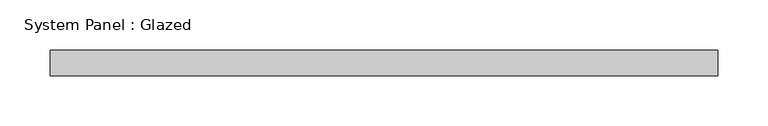
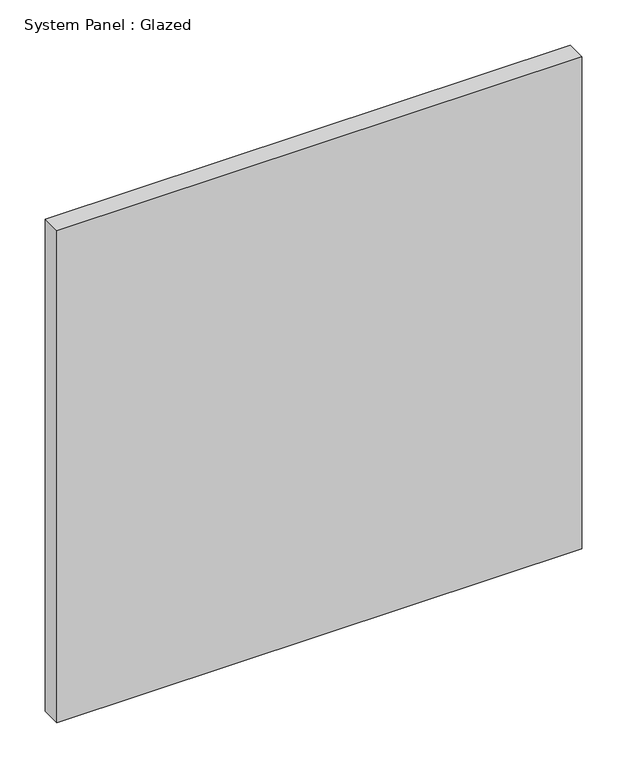
"""IFC4 building model written with IfcOpenShell, lengths in millimetres: plate geometry, System Panel : Glazed."""

from ifc_helpers import new_model, si_unit, origin, origin_with_axes, place, context, project, spatial, polyline, outline, extrude, source, transform, mapped, element, save


def system_panel_glazed_687c427d(model_context):
    return source(origin(), model_context, "Body", "SweptSolid", [
        extrude(outline(polyline([(333.375, 19.05), (-333.375, 19.05), (-333.375, 44.45), (333.375, 44.45), (333.375, 19.05)])), origin_with_axes(), (0.0, 0.0, 1.0), 661.0861093),
    ])


if __name__ == "__main__":
    model = new_model("IFC4")
    model_context = context("Model", 3, world=origin())
    ifc_project = project(units=[si_unit("LENGTHUNIT", "METRE", prefix="MILLI")], contexts=[model_context])
    site = spatial("IfcSite", under=ifc_project)
    building = spatial("IfcBuilding", under=site)
    placement = place(None, origin())
    system_panel_glazed_shape = system_panel_glazed_687c427d(model_context)
    element("IfcPlate", 1, ObjectType="System Panel : Glazed", at=placement, inside=building, context=model_context, shape_type="MappedRepresentation", body=[
        mapped(system_panel_glazed_shape, transform((0.0, 0.0, 0.0), x_axis=(1.0, 0.0, 0.0), y_axis=(0.0, 1.0, 0.0), z_axis=(0.0, 0.0, 1.0))),
    ])
    save(model, "model.ifc")

# Revit data of these elements
# Type "System Panel : Glazed"
#   Construction Type Id = "GSP4R"
#   Analytic Construction = "1/8 in Pilkington single glazing"
#   Visual Light Transmittance = 0.9
#   Solar Heat Gain Coefficient = 0.86
#   Heat Transfer Coefficient (U) = 1.18115 BTU/(h·ft²·°F)
#   Define Thermal Properties by = 1
# Element 1 (IfcPlate, "System Panel : Glazed")
#   Materials on its faces: "Glass"
# Materials
#   "Glass": class "Glass", colour RGB 0 128 192, transparency 0.75, Description = "Soda Lime Glass", Cost = 0
